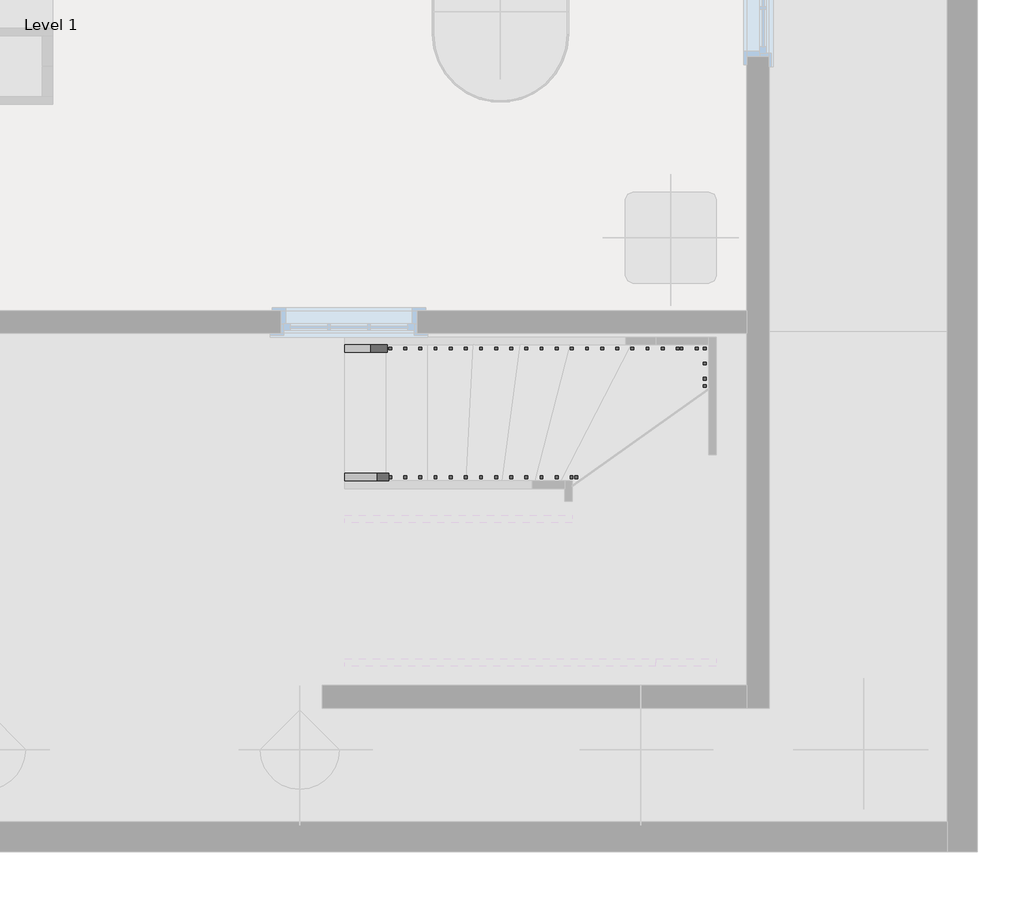
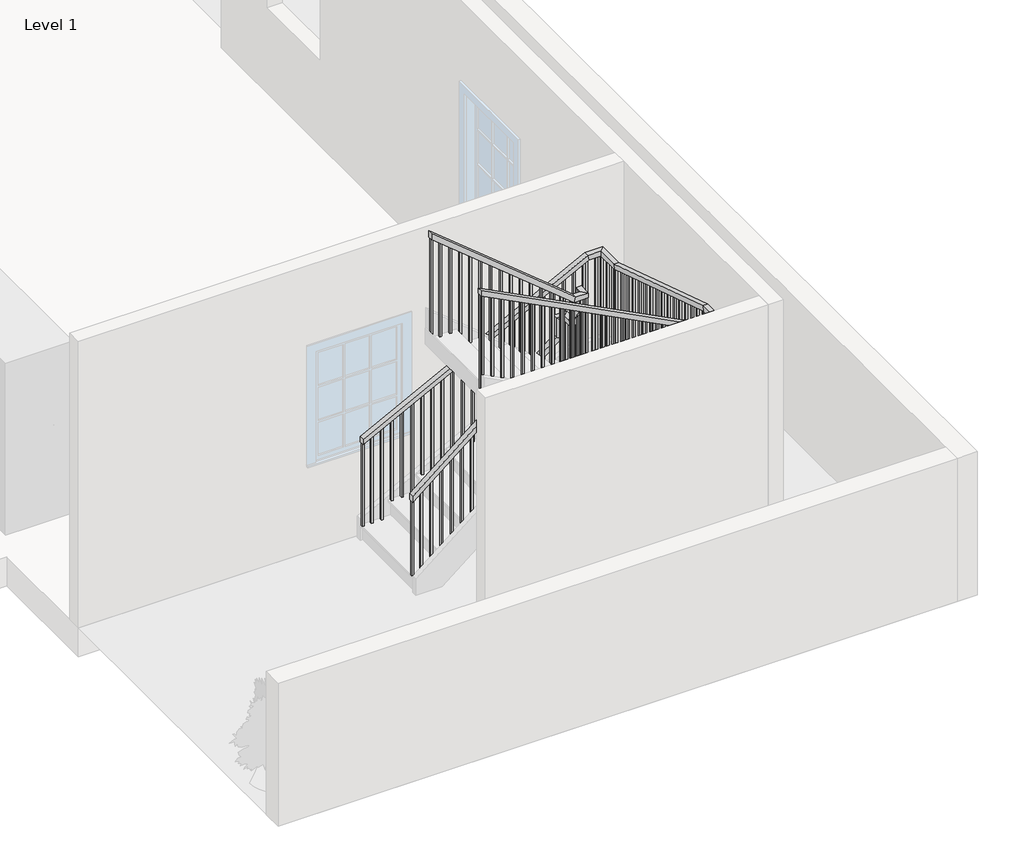
# One storey, part 2 of 3: 2 railings.
"""IFC4 building model written with IfcOpenShell, lengths in millimetres."""

from ifc_helpers import new_model, si_unit, frame, origin, place, context, project, spatial, polyline, outline, extrude, faceted_brep, element, save

model = new_model("IFC4")

# Units and contexts
model_context = context("Model", 3, world=origin())
ifc_project = project(units=[si_unit("LENGTHUNIT", "METRE", prefix="MILLI")], contexts=[model_context])

# Site, building, storey
site = spatial("IfcSite", under=ifc_project)
building = spatial("IfcBuilding", under=site)
storey = spatial("IfcBuildingStorey", under=building, Name="Level 1", Elevation=0.0)

# Railings
placement = place(None, origin())
element("IfcRailing", 1, ObjectType="Handrail - Rectangular", at=placement, inside=storey, context=model_context, shape_type="SolidModel", body=[
    faceted_brep([(-3966.7570938, 433.3007235, 1025.2529681), (-3966.7570938, 433.3007235, 959.7067088), (-3966.7570938, 382.5007235, 959.7067088), (-3966.7570938, 382.5007235, 1025.2529681), (-2515.2254019, 433.3007235, 2208.7848338), (-2464.4254019, 433.3007235, 2184.659247), (-2464.4254019, 382.5007235, 2184.659247), (-2515.2254019, 382.5007235, 2208.7848338), (-2515.2254019, 433.3007235, 2414.6281882), (-2464.4254019, 433.3007235, 2363.8281882), (-2464.4254019, 382.5007235, 2363.8281882), (-2515.2254019, 382.5007235, 2414.6281882), (-2388.2254019, 433.3007235, 2414.6281882), (-2388.2254019, 433.3007235, 2363.8281882), (-2439.0254019, 382.5007235, 2363.8281882), (-2439.0254019, 382.5007235, 2414.6281882), (-2388.2254019, 306.3007235, 2414.6281882), (-2388.2254019, 277.1793897, 2363.8281882), (-2439.0254019, 277.1793897, 2363.8281882), (-2439.0254019, 306.3007235, 2414.6281882), (-2388.2254019, 179.3007235, 2631.5051451), (-2388.2254019, 128.5007235, 2617.7256424), (-2439.0254019, 128.5007235, 2617.7256424), (-2439.0254019, 179.3007235, 2631.5051451), (-2388.2254019, 179.3007235, 2837.3484995), (-2388.2254019, 128.5007235, 2786.5484995), (-2439.0254019, 128.5007235, 2786.5484995), (-2439.0254019, 179.3007235, 2837.3484995), (-2388.2254019, 52.3007235, 2837.3484995), (-2388.2254019, 52.3007235, 2786.5484995), (-2439.0254019, 103.1007235, 2786.5484995), (-2439.0254019, 103.1007235, 2837.3484995), (-2515.2254019, 52.3007235, 2837.3484995), (-2533.310815, 52.3007235, 2786.5484995), (-2533.310815, 103.1007235, 2786.5484995), (-2515.2254019, 103.1007235, 2837.3484995), (-3966.7570938, 52.3007235, 4020.8803652), (-3966.7570938, 103.1007235, 4020.8803652), (-3966.7570938, 103.1007235, 3955.3341059), (-3966.7570938, 52.3007235, 3955.3341059)], [[[0, 1, 2, 3]], [[1, 0, 4, 5]], [[2, 1, 5, 6]], [[3, 2, 6, 7]], [[0, 3, 7, 4]], [[5, 4, 8, 9]], [[6, 5, 9, 10]], [[7, 6, 10, 11]], [[4, 7, 11, 8]], [[9, 8, 12, 13]], [[10, 9, 13, 14]], [[11, 10, 14, 15]], [[8, 11, 15, 12]], [[13, 12, 16, 17]], [[14, 13, 17, 18]], [[15, 14, 18, 19]], [[12, 15, 19, 16]], [[17, 16, 20, 21]], [[18, 17, 21, 22]], [[19, 18, 22, 23]], [[16, 19, 23, 20]], [[21, 20, 24, 25]], [[22, 21, 25, 26]], [[23, 22, 26, 27]], [[20, 23, 27, 24]], [[25, 24, 28, 29]], [[26, 25, 29, 30]], [[27, 26, 30, 31]], [[24, 27, 31, 28]], [[29, 28, 32, 33]], [[30, 29, 33, 34]], [[31, 30, 34, 35]], [[28, 31, 35, 32]], [[36, 37, 38, 39]], [[33, 32, 36, 39]], [[34, 33, 39, 38]], [[35, 34, 38, 37]], [[32, 35, 37, 36]]]),
    extrude(outline(polyline([(3866.2231262, -3857.4677583), (3881.7558784, -3876.5177583), (2878.6666667, -3876.5177583), (2878.6666667, -3857.4677583), (3866.2231262, -3857.4677583)])), frame((0.0, 68.1757235, 0.0), z_axis=(0.0, 1.0, 0.0), x_axis=(0.0, 0.0, 1.0)), (0.0, 0.0, 1.0), 19.05),
    extrude(outline(polyline([(3783.3817813, -3755.8677583), (3798.9145334, -3774.9177583), (2878.6666667, -3774.9177583), (2878.6666667, -3755.8677583), (3783.3817813, -3755.8677583)])), frame((0.0, 68.1757235, 0.0), z_axis=(0.0, 1.0, 0.0), x_axis=(0.0, 0.0, 1.0)), (0.0, 0.0, 1.0), 19.05),
    extrude(outline(polyline([(3700.5404364, -3654.2677583), (3716.0731885, -3673.3177583), (2709.3333333, -3673.3177583), (2709.3333333, -3654.2677583), (3700.5404364, -3654.2677583)])), frame((0.0, 68.1757235, 0.0), z_axis=(0.0, 1.0, 0.0), x_axis=(0.0, 0.0, 1.0)), (0.0, 0.0, 1.0), 19.05),
    extrude(outline(polyline([(3617.6990914, -3552.6677583), (3633.2318436, -3571.7177583), (2709.3333333, -3571.7177583), (2709.3333333, -3552.6677583), (3617.6990914, -3552.6677583)])), frame((0.0, 68.1757235, 0.0), z_axis=(0.0, 1.0, 0.0), x_axis=(0.0, 0.0, 1.0)), (0.0, 0.0, 1.0), 19.05),
    extrude(outline(polyline([(3534.8577465, -3451.0677583), (3550.3904987, -3470.1177583), (2709.3333333, -3470.1177583), (2709.3333333, -3451.0677583), (3534.8577465, -3451.0677583)])), frame((0.0, 68.1757235, 0.0), z_axis=(0.0, 1.0, 0.0), x_axis=(0.0, 0.0, 1.0)), (0.0, 0.0, 1.0), 19.05),
    extrude(outline(polyline([(3452.0164016, -3349.4677583), (3467.5491538, -3368.5177583), (2540.0, -3368.5177583), (2540.0, -3349.4677583), (3452.0164016, -3349.4677583)])), frame((0.0, 68.1757235, 0.0), z_axis=(0.0, 1.0, 0.0), x_axis=(0.0, 0.0, 1.0)), (0.0, 0.0, 1.0), 19.05),
    extrude(outline(polyline([(3369.1750567, -3247.8677583), (3384.7078088, -3266.9177583), (2540.0, -3266.9177583), (2540.0, -3247.8677583), (3369.1750567, -3247.8677583)])), frame((0.0, 68.1757235, 0.0), z_axis=(0.0, 1.0, 0.0), x_axis=(0.0, 0.0, 1.0)), (0.0, 0.0, 1.0), 19.05),
    extrude(outline(polyline([(3286.3337117, -3146.2677583), (3301.8664639, -3165.3177583), (2540.0, -3165.3177583), (2540.0, -3146.2677583), (3286.3337117, -3146.2677583)])), frame((0.0, 68.1757235, 0.0), z_axis=(0.0, 1.0, 0.0), x_axis=(0.0, 0.0, 1.0)), (0.0, 0.0, 1.0), 19.05),
    extrude(outline(polyline([(3203.4923668, -3044.6677583), (3219.025119, -3063.7177583), (2370.6666667, -3063.7177583), (2370.6666667, -3044.6677583), (3203.4923668, -3044.6677583)])), frame((0.0, 68.1757235, 0.0), z_axis=(0.0, 1.0, 0.0), x_axis=(0.0, 0.0, 1.0)), (0.0, 0.0, 1.0), 19.05),
    extrude(outline(polyline([(3120.6510219, -2943.0677583), (3136.1837741, -2962.1177583), (2370.6666667, -2962.1177583), (2370.6666667, -2943.0677583), (3120.6510219, -2943.0677583)])), frame((0.0, 68.1757235, 0.0), z_axis=(0.0, 1.0, 0.0), x_axis=(0.0, 0.0, 1.0)), (0.0, 0.0, 1.0), 19.05),
    extrude(outline(polyline([(3037.809677, -2841.4677583), (3053.3424291, -2860.5177583), (2201.3333333, -2860.5177583), (2201.3333333, -2841.4677583), (3037.809677, -2841.4677583)])), frame((0.0, 68.1757235, 0.0), z_axis=(0.0, 1.0, 0.0), x_axis=(0.0, 0.0, 1.0)), (0.0, 0.0, 1.0), 19.05),
    extrude(outline(polyline([(2954.9683321, -2739.8677583), (2970.5010842, -2758.9177583), (2201.3333333, -2758.9177583), (2201.3333333, -2739.8677583), (2954.9683321, -2739.8677583)])), frame((0.0, 68.1757235, 0.0), z_axis=(0.0, 1.0, 0.0), x_axis=(0.0, 0.0, 1.0)), (0.0, 0.0, 1.0), 19.05),
    extrude(outline(polyline([(2872.1269871, -2638.2677583), (2887.6597393, -2657.3177583), (2032.0, -2657.3177583), (2032.0, -2638.2677583), (2872.1269871, -2638.2677583)])), frame((0.0, 68.1757235, 0.0), z_axis=(0.0, 1.0, 0.0), x_axis=(0.0, 0.0, 1.0)), (0.0, 0.0, 1.0), 19.05),
    extrude(outline(polyline([(2789.2856422, -2536.6677583), (2804.8183944, -2555.7177583), (2032.0, -2555.7177583), (2032.0, -2536.6677583), (2789.2856422, -2536.6677583)])), frame((0.0, 68.1757235, 0.0), z_axis=(0.0, 1.0, 0.0), x_axis=(0.0, 0.0, 1.0)), (0.0, 0.0, 1.0), 19.05),
    extrude(outline(polyline([(180.3898197, 2529.115018), (199.4398197, 2496.5834745), (199.4398197, 1524.0), (180.3898197, 1524.0), (180.3898197, 2529.115018)])), frame((-2423.1504019, 0.0, 0.0), z_axis=(1.0, 0.0, 0.0), x_axis=(0.0, 1.0, 0.0)), (0.0, 0.0, 1.0), 19.05),
    extrude(outline(polyline([(281.9898197, 2355.6134525), (301.0398197, 2323.0819089), (301.0398197, 1524.0), (281.9898197, 1524.0), (281.9898197, 2355.6134525)])), frame((-2423.1504019, 0.0, 0.0), z_axis=(1.0, 0.0, 0.0), x_axis=(0.0, 1.0, 0.0)), (0.0, 0.0, 1.0), 19.05),
    extrude(outline(polyline([(2127.2519138, -2534.8320938), (2111.7191617, -2553.8820938), (1016.0, -2553.8820938), (1016.0, -2534.8320938), (2127.2519138, -2534.8320938)])), frame((0.0, 398.3757235, 0.0), z_axis=(0.0, 1.0, 0.0), x_axis=(0.0, 0.0, 1.0)), (0.0, 0.0, 1.0), 19.05),
    extrude(outline(polyline([(2044.4105689, -2636.4320938), (2028.8778167, -2655.4820938), (1016.0, -2655.4820938), (1016.0, -2636.4320938), (2044.4105689, -2636.4320938)])), frame((0.0, 398.3757235, 0.0), z_axis=(0.0, 1.0, 0.0), x_axis=(0.0, 0.0, 1.0)), (0.0, 0.0, 1.0), 19.05),
    extrude(outline(polyline([(1961.569224, -2738.0320938), (1946.0364718, -2757.0820938), (846.6666667, -2757.0820938), (846.6666667, -2738.0320938), (1961.569224, -2738.0320938)])), frame((0.0, 398.3757235, 0.0), z_axis=(0.0, 1.0, 0.0), x_axis=(0.0, 0.0, 1.0)), (0.0, 0.0, 1.0), 19.05),
    extrude(outline(polyline([(1878.7278791, -2839.6320938), (1863.1951269, -2858.6820938), (846.6666667, -2858.6820938), (846.6666667, -2839.6320938), (1878.7278791, -2839.6320938)])), frame((0.0, 398.3757235, 0.0), z_axis=(0.0, 1.0, 0.0), x_axis=(0.0, 0.0, 1.0)), (0.0, 0.0, 1.0), 19.05),
    extrude(outline(polyline([(1795.8865341, -2941.2320938), (1780.353782, -2960.2820938), (677.3333333, -2960.2820938), (677.3333333, -2941.2320938), (1795.8865341, -2941.2320938)])), frame((0.0, 398.3757235, 0.0), z_axis=(0.0, 1.0, 0.0), x_axis=(0.0, 0.0, 1.0)), (0.0, 0.0, 1.0), 19.05),
    extrude(outline(polyline([(1713.0451892, -3042.8320938), (1697.5124371, -3061.8820938), (677.3333333, -3061.8820938), (677.3333333, -3042.8320938), (1713.0451892, -3042.8320938)])), frame((0.0, 398.3757235, 0.0), z_axis=(0.0, 1.0, 0.0), x_axis=(0.0, 0.0, 1.0)), (0.0, 0.0, 1.0), 19.05),
    extrude(outline(polyline([(1630.2038443, -3144.4320938), (1614.6710921, -3163.4820938), (508.0, -3163.4820938), (508.0, -3144.4320938), (1630.2038443, -3144.4320938)])), frame((0.0, 398.3757235, 0.0), z_axis=(0.0, 1.0, 0.0), x_axis=(0.0, 0.0, 1.0)), (0.0, 0.0, 1.0), 19.05),
    extrude(outline(polyline([(1547.3624994, -3246.0320938), (1531.8297472, -3265.0820938), (508.0, -3265.0820938), (508.0, -3246.0320938), (1547.3624994, -3246.0320938)])), frame((0.0, 398.3757235, 0.0), z_axis=(0.0, 1.0, 0.0), x_axis=(0.0, 0.0, 1.0)), (0.0, 0.0, 1.0), 19.05),
    extrude(outline(polyline([(1464.5211545, -3347.6320938), (1448.9884023, -3366.6820938), (508.0, -3366.6820938), (508.0, -3347.6320938), (1464.5211545, -3347.6320938)])), frame((0.0, 398.3757235, 0.0), z_axis=(0.0, 1.0, 0.0), x_axis=(0.0, 0.0, 1.0)), (0.0, 0.0, 1.0), 19.05),
    extrude(outline(polyline([(1381.6798095, -3449.2320938), (1366.1470574, -3468.2820938), (338.6666667, -3468.2820938), (338.6666667, -3449.2320938), (1381.6798095, -3449.2320938)])), frame((0.0, 398.3757235, 0.0), z_axis=(0.0, 1.0, 0.0), x_axis=(0.0, 0.0, 1.0)), (0.0, 0.0, 1.0), 19.05),
    extrude(outline(polyline([(1298.8384646, -3550.8320938), (1283.3057124, -3569.8820938), (338.6666667, -3569.8820938), (338.6666667, -3550.8320938), (1298.8384646, -3550.8320938)])), frame((0.0, 398.3757235, 0.0), z_axis=(0.0, 1.0, 0.0), x_axis=(0.0, 0.0, 1.0)), (0.0, 0.0, 1.0), 19.05),
    extrude(outline(polyline([(1215.9971197, -3652.4320938), (1200.4643675, -3671.4820938), (338.6666667, -3671.4820938), (338.6666667, -3652.4320938), (1215.9971197, -3652.4320938)])), frame((0.0, 398.3757235, 0.0), z_axis=(0.0, 1.0, 0.0), x_axis=(0.0, 0.0, 1.0)), (0.0, 0.0, 1.0), 19.05),
    extrude(outline(polyline([(1133.1557748, -3754.0320938), (1117.6230226, -3773.0820938), (169.3333333, -3773.0820938), (169.3333333, -3754.0320938), (1133.1557748, -3754.0320938)])), frame((0.0, 398.3757235, 0.0), z_axis=(0.0, 1.0, 0.0), x_axis=(0.0, 0.0, 1.0)), (0.0, 0.0, 1.0), 19.05),
    extrude(outline(polyline([(1050.3144298, -3855.6320938), (1034.7816777, -3874.6820938), (169.3333333, -3874.6820938), (169.3333333, -3855.6320938), (1050.3144298, -3855.6320938)])), frame((0.0, 398.3757235, 0.0), z_axis=(0.0, 1.0, 0.0), x_axis=(0.0, 0.0, 1.0)), (0.0, 0.0, 1.0), 19.05),
    extrude(outline(polyline([(-2435.0677583, 87.2257235), (-2435.0677583, 68.1757235), (-2454.1177583, 68.1757235), (-2454.1177583, 87.2257235), (-2435.0677583, 87.2257235)])), frame((0.0, 0.0, 1862.6666667), z_axis=(0.0, 0.0, 1.0), x_axis=(1.0, 0.0, 0.0)), (0.0, 0.0, 1.0), 923.8818329),
    extrude(outline(polyline([(-2423.1504019, 87.2257235), (-2404.1004019, 87.2257235), (-2404.1004019, 68.1757235), (-2423.1504019, 68.1757235), (-2423.1504019, 87.2257235)])), frame((0.0, 0.0, 1862.6666667), z_axis=(0.0, 0.0, 1.0), x_axis=(1.0, 0.0, 0.0)), (0.0, 0.0, 1.0), 923.8818329),
    extrude(outline(polyline([(-2423.1504019, 102.0116273), (-2404.1004019, 102.0116273), (-2404.1004019, 82.9616273), (-2423.1504019, 82.9616273), (-2423.1504019, 102.0116273)])), frame((0.0, 0.0, 1693.3333333), z_axis=(0.0, 0.0, 1.0), x_axis=(1.0, 0.0, 0.0)), (0.0, 0.0, 1.0), 1093.2151662),
    extrude(outline(polyline([(-2423.1504019, 402.6398197), (-2404.1004019, 402.6398197), (-2404.1004019, 383.5898197), (-2423.1504019, 383.5898197), (-2423.1504019, 402.6398197)])), frame((0.0, 0.0, 1354.6666667), z_axis=(0.0, 0.0, 1.0), x_axis=(1.0, 0.0, 0.0)), (0.0, 0.0, 1.0), 1009.1615215),
    extrude(outline(polyline([(-2423.1504019, 398.3757235), (-2423.1504019, 417.4257235), (-2404.1004019, 417.4257235), (-2404.1004019, 398.3757235), (-2423.1504019, 398.3757235)])), frame((0.0, 0.0, 1185.3333333), z_axis=(0.0, 0.0, 1.0), x_axis=(1.0, 0.0, 0.0)), (0.0, 0.0, 1.0), 1178.4948549),
    extrude(outline(polyline([(-2454.1177583, 398.3757235), (-2454.1177583, 417.4257235), (-2435.0677583, 417.4257235), (-2435.0677583, 398.3757235), (-2454.1177583, 398.3757235)])), frame((0.0, 0.0, 1185.3333333), z_axis=(0.0, 0.0, 1.0), x_axis=(1.0, 0.0, 0.0)), (0.0, 0.0, 1.0), 1178.4948549),
    extrude(outline(polyline([(3939.8013537, -3947.7070938), (3955.3341059, -3966.7570938), (2878.6666667, -3966.7570938), (2878.6666667, -3947.7070938), (3939.8013537, -3947.7070938)])), frame((0.0, 68.1757235, 0.0), z_axis=(0.0, 1.0, 0.0), x_axis=(0.0, 0.0, 1.0)), (0.0, 0.0, 1.0), 19.05),
    extrude(outline(polyline([(975.239461, -3947.7070938), (959.7067088, -3966.7570938), (169.3333333, -3966.7570938), (169.3333333, -3947.7070938), (975.239461, -3947.7070938)])), frame((0.0, 398.3757235, 0.0), z_axis=(0.0, 1.0, 0.0), x_axis=(0.0, 0.0, 1.0)), (0.0, 0.0, 1.0), 19.05),
])
element("IfcRailing", 2, ObjectType="Handrail - Rectangular", at=placement, inside=storey, context=model_context, shape_type="SolidModel", body=[
    faceted_brep([(-3966.7570938, 1296.9007235, 1109.0771751), (-3966.7570938, 1296.9007235, 1051.9280057), (-3966.7570938, 1246.1007235, 1051.9280057), (-3966.7570938, 1246.1007235, 1109.0771751), (-1706.7752373, 1296.9007235, 2273.7644996), (-1694.455186, 1296.9007235, 2222.9644996), (-1694.455186, 1246.1007235, 2222.9644996), (-1706.7752373, 1246.1007235, 2273.7644996), (-1524.6254019, 1296.9007235, 2273.7644996), (-1524.6254019, 1296.9007235, 2222.9644996), (-1575.4254019, 1246.1007235, 2222.9644996), (-1575.4254019, 1246.1007235, 2273.7644996), (-1524.6254019, 1019.7467709, 2273.7644996), (-1524.6254019, 1011.7961947, 2222.9644996), (-1575.4254019, 1011.7961947, 2222.9644996), (-1575.4254019, 1019.7467709, 2273.7644996), (-1524.6254019, -534.1453239, 2772.3688337), (-1524.6254019, -542.0959, 2721.5688337), (-1575.4254019, -542.0959, 2721.5688337), (-1575.4254019, -534.1453239, 2772.3688337), (-1524.6254019, -811.2992765, 2772.3688337), (-1524.6254019, -811.2992765, 2721.5688337), (-1575.4254019, -760.4992765, 2721.5688337), (-1575.4254019, -760.4992765, 2772.3688337), (-1706.7752373, -811.2992765, 2772.3688337), (-1719.0952886, -811.2992765, 2721.5688337), (-1719.0952886, -760.4992765, 2721.5688337), (-1706.7752373, -760.4992765, 2772.3688337), (-3966.7570938, -811.2992765, 3937.0561582), (-3966.7570938, -760.4992765, 3937.0561582), (-3966.7570938, -760.4992765, 3879.9069889), (-3966.7570938, -811.2992765, 3879.9069889)], [[[0, 1, 2, 3]], [[1, 0, 4, 5]], [[2, 1, 5, 6]], [[3, 2, 6, 7]], [[0, 3, 7, 4]], [[5, 4, 8, 9]], [[6, 5, 9, 10]], [[7, 6, 10, 11]], [[4, 7, 11, 8]], [[9, 8, 12, 13]], [[10, 9, 13, 14]], [[11, 10, 14, 15]], [[8, 11, 15, 12]], [[13, 12, 16, 17]], [[14, 13, 17, 18]], [[15, 14, 18, 19]], [[12, 15, 19, 16]], [[17, 16, 20, 21]], [[18, 17, 21, 22]], [[19, 18, 22, 23]], [[16, 19, 23, 20]], [[21, 20, 24, 25]], [[22, 21, 25, 26]], [[23, 22, 26, 27]], [[20, 23, 27, 24]], [[28, 29, 30, 31]], [[25, 24, 28, 31]], [[26, 25, 31, 30]], [[27, 26, 30, 29]], [[24, 27, 29, 28]]]),
    extrude(outline(polyline([(3872.0443296, -3951.5002373), (2878.6666667, -3951.5002373), (2878.6666667, -3932.4502373), (3862.2268642, -3932.4502373), (3872.0443296, -3951.5002373)])), frame((0.0, -795.4242765, 0.0), z_axis=(0.0, 1.0, 0.0), x_axis=(0.0, 0.0, 1.0)), (0.0, 0.0, 1.0), 19.05),
    extrude(outline(polyline([(3819.6845145, -3849.9002373), (2878.6666667, -3849.9002373), (2878.6666667, -3830.8502373), (3809.8670491, -3830.8502373), (3819.6845145, -3849.9002373)])), frame((0.0, -795.4242765, 0.0), z_axis=(0.0, 1.0, 0.0), x_axis=(0.0, 0.0, 1.0)), (0.0, 0.0, 1.0), 19.05),
    extrude(outline(polyline([(3767.3246993, -3748.3002373), (2878.6666667, -3748.3002373), (2878.6666667, -3729.2502373), (3757.507234, -3729.2502373), (3767.3246993, -3748.3002373)])), frame((0.0, -795.4242765, 0.0), z_axis=(0.0, 1.0, 0.0), x_axis=(0.0, 0.0, 1.0)), (0.0, 0.0, 1.0), 19.05),
    extrude(outline(polyline([(3714.9648842, -3646.7002373), (2709.3333333, -3646.7002373), (2709.3333333, -3627.6502373), (3705.1474189, -3627.6502373), (3714.9648842, -3646.7002373)])), frame((0.0, -795.4242765, 0.0), z_axis=(0.0, 1.0, 0.0), x_axis=(0.0, 0.0, 1.0)), (0.0, 0.0, 1.0), 19.05),
    extrude(outline(polyline([(3662.6050691, -3545.1002373), (2709.3333333, -3545.1002373), (2709.3333333, -3526.0502373), (3652.7876038, -3526.0502373), (3662.6050691, -3545.1002373)])), frame((0.0, -795.4242765, 0.0), z_axis=(0.0, 1.0, 0.0), x_axis=(0.0, 0.0, 1.0)), (0.0, 0.0, 1.0), 19.05),
    extrude(outline(polyline([(3610.245254, -3443.5002373), (2709.3333333, -3443.5002373), (2709.3333333, -3424.4502373), (3600.4277887, -3424.4502373), (3610.245254, -3443.5002373)])), frame((0.0, -795.4242765, 0.0), z_axis=(0.0, 1.0, 0.0), x_axis=(0.0, 0.0, 1.0)), (0.0, 0.0, 1.0), 19.05),
    extrude(outline(polyline([(3557.8854389, -3341.9002373), (2540.0, -3341.9002373), (2540.0, -3322.8502373), (3548.0679735, -3322.8502373), (3557.8854389, -3341.9002373)])), frame((0.0, -795.4242765, 0.0), z_axis=(0.0, 1.0, 0.0), x_axis=(0.0, 0.0, 1.0)), (0.0, 0.0, 1.0), 19.05),
    extrude(outline(polyline([(3505.5256238, -3240.3002373), (2540.0, -3240.3002373), (2540.0, -3221.2502373), (3495.7081584, -3221.2502373), (3505.5256238, -3240.3002373)])), frame((0.0, -795.4242765, 0.0), z_axis=(0.0, 1.0, 0.0), x_axis=(0.0, 0.0, 1.0)), (0.0, 0.0, 1.0), 19.05),
    extrude(outline(polyline([(3453.1658086, -3138.7002373), (2540.0, -3138.7002373), (2540.0, -3119.6502373), (3443.3483433, -3119.6502373), (3453.1658086, -3138.7002373)])), frame((0.0, -795.4242765, 0.0), z_axis=(0.0, 1.0, 0.0), x_axis=(0.0, 0.0, 1.0)), (0.0, 0.0, 1.0), 19.05),
    extrude(outline(polyline([(3400.8059935, -3037.1002373), (2370.6666667, -3037.1002373), (2370.6666667, -3018.0502373), (3390.9885282, -3018.0502373), (3400.8059935, -3037.1002373)])), frame((0.0, -795.4242765, 0.0), z_axis=(0.0, 1.0, 0.0), x_axis=(0.0, 0.0, 1.0)), (0.0, 0.0, 1.0), 19.05),
    extrude(outline(polyline([(3348.4461784, -2935.5002373), (2370.6666667, -2935.5002373), (2370.6666667, -2916.4502373), (3338.6287131, -2916.4502373), (3348.4461784, -2935.5002373)])), frame((0.0, -795.4242765, 0.0), z_axis=(0.0, 1.0, 0.0), x_axis=(0.0, 0.0, 1.0)), (0.0, 0.0, 1.0), 19.05),
    extrude(outline(polyline([(3296.0863633, -2833.9002373), (2370.6666667, -2833.9002373), (2370.6666667, -2814.8502373), (3286.268898, -2814.8502373), (3296.0863633, -2833.9002373)])), frame((0.0, -795.4242765, 0.0), z_axis=(0.0, 1.0, 0.0), x_axis=(0.0, 0.0, 1.0)), (0.0, 0.0, 1.0), 19.05),
    extrude(outline(polyline([(3243.7265482, -2732.3002373), (2201.3333333, -2732.3002373), (2201.3333333, -2713.2502373), (3233.9090828, -2713.2502373), (3243.7265482, -2732.3002373)])), frame((0.0, -795.4242765, 0.0), z_axis=(0.0, 1.0, 0.0), x_axis=(0.0, 0.0, 1.0)), (0.0, 0.0, 1.0), 19.05),
    extrude(outline(polyline([(3191.3667331, -2630.7002373), (2201.3333333, -2630.7002373), (2201.3333333, -2611.6502373), (3181.5492677, -2611.6502373), (3191.3667331, -2630.7002373)])), frame((0.0, -795.4242765, 0.0), z_axis=(0.0, 1.0, 0.0), x_axis=(0.0, 0.0, 1.0)), (0.0, 0.0, 1.0), 19.05),
    extrude(outline(polyline([(3139.0069179, -2529.1002373), (2201.3333333, -2529.1002373), (2201.3333333, -2510.0502373), (3129.1894526, -2510.0502373), (3139.0069179, -2529.1002373)])), frame((0.0, -795.4242765, 0.0), z_axis=(0.0, 1.0, 0.0), x_axis=(0.0, 0.0, 1.0)), (0.0, 0.0, 1.0), 19.05),
    extrude(outline(polyline([(3086.6471028, -2427.5002373), (2032.0, -2427.5002373), (2032.0, -2408.4502373), (3076.8296375, -2408.4502373), (3086.6471028, -2427.5002373)])), frame((0.0, -795.4242765, 0.0), z_axis=(0.0, 1.0, 0.0), x_axis=(0.0, 0.0, 1.0)), (0.0, 0.0, 1.0), 19.05),
    extrude(outline(polyline([(3034.2872877, -2325.9002373), (2032.0, -2325.9002373), (2032.0, -2306.8502373), (3024.4698224, -2306.8502373), (3034.2872877, -2325.9002373)])), frame((0.0, -795.4242765, 0.0), z_axis=(0.0, 1.0, 0.0), x_axis=(0.0, 0.0, 1.0)), (0.0, 0.0, 1.0), 19.05),
    extrude(outline(polyline([(2981.9274726, -2224.3002373), (2032.0, -2224.3002373), (2032.0, -2205.2502373), (2972.1100073, -2205.2502373), (2981.9274726, -2224.3002373)])), frame((0.0, -795.4242765, 0.0), z_axis=(0.0, 1.0, 0.0), x_axis=(0.0, 0.0, 1.0)), (0.0, 0.0, 1.0), 19.05),
    extrude(outline(polyline([(2929.5676575, -2122.7002373), (2032.0, -2122.7002373), (2032.0, -2103.6502373), (2919.7501921, -2103.6502373), (2929.5676575, -2122.7002373)])), frame((0.0, -795.4242765, 0.0), z_axis=(0.0, 1.0, 0.0), x_axis=(0.0, 0.0, 1.0)), (0.0, 0.0, 1.0), 19.05),
    extrude(outline(polyline([(2877.2078424, -2021.1002373), (1862.6666667, -2021.1002373), (1862.6666667, -2002.0502373), (2867.390377, -2002.0502373), (2877.2078424, -2021.1002373)])), frame((0.0, -795.4242765, 0.0), z_axis=(0.0, 1.0, 0.0), x_axis=(0.0, 0.0, 1.0)), (0.0, 0.0, 1.0), 19.05),
    extrude(outline(polyline([(2824.8480272, -1919.5002373), (1862.6666667, -1919.5002373), (1862.6666667, -1900.4502373), (2815.0305619, -1900.4502373), (2824.8480272, -1919.5002373)])), frame((0.0, -795.4242765, 0.0), z_axis=(0.0, 1.0, 0.0), x_axis=(0.0, 0.0, 1.0)), (0.0, 0.0, 1.0), 19.05),
    extrude(outline(polyline([(2772.4882121, -1817.9002373), (1862.6666667, -1817.9002373), (1862.6666667, -1798.8502373), (2762.6707468, -1798.8502373), (2772.4882121, -1817.9002373)])), frame((0.0, -795.4242765, 0.0), z_axis=(0.0, 1.0, 0.0), x_axis=(0.0, 0.0, 1.0)), (0.0, 0.0, 1.0), 19.05),
    extrude(outline(polyline([(-1642.1004019, -795.4242765), (-1661.1504019, -795.4242765), (-1661.1504019, -776.3742765), (-1642.1004019, -776.3742765), (-1642.1004019, -795.4242765)])), frame((0.0, 0.0, 1862.6666667), z_axis=(0.0, 0.0, 1.0), x_axis=(1.0, 0.0, 0.0)), (0.0, 0.0, 1.0), 858.902167),
    extrude(outline(polyline([(-1540.5004019, -727.8203239), (-1540.5004019, -746.8703239), (-1559.5504019, -746.8703239), (-1559.5504019, -727.8203239), (-1540.5004019, -727.8203239)])), frame((0.0, 0.0, 1862.6666667), z_axis=(0.0, 0.0, 1.0), x_axis=(1.0, 0.0, 0.0)), (0.0, 0.0, 1.0), 858.902167),
    extrude(outline(polyline([(-1540.5004019, -626.2203239), (-1540.5004019, -645.2703239), (-1559.5504019, -645.2703239), (-1559.5504019, -626.2203239), (-1540.5004019, -626.2203239)])), frame((0.0, 0.0, 1862.6666667), z_axis=(0.0, 0.0, 1.0), x_axis=(1.0, 0.0, 0.0)), (0.0, 0.0, 1.0), 858.902167),
    extrude(outline(polyline([(-494.7282291, 2706.3697564), (-494.7282291, 1693.3333333), (-513.7782291, 1693.3333333), (-513.7782291, 2712.4824155), (-494.7282291, 2706.3697564)])), frame((-1559.5504019, 0.0, 0.0), z_axis=(1.0, 0.0, 0.0), x_axis=(0.0, 1.0, 0.0)), (0.0, 0.0, 1.0), 19.05),
    extrude(outline(polyline([(-393.1282291, 2673.7689082), (-393.1282291, 1693.3333333), (-412.1782291, 1693.3333333), (-412.1782291, 2679.8815673), (-393.1282291, 2673.7689082)])), frame((-1559.5504019, 0.0, 0.0), z_axis=(1.0, 0.0, 0.0), x_axis=(0.0, 1.0, 0.0)), (0.0, 0.0, 1.0), 19.05),
    extrude(outline(polyline([(-291.5282291, 2641.16806), (-291.5282291, 1693.3333333), (-310.5782291, 1693.3333333), (-310.5782291, 2647.280719), (-291.5282291, 2641.16806)])), frame((-1559.5504019, 0.0, 0.0), z_axis=(1.0, 0.0, 0.0), x_axis=(0.0, 1.0, 0.0)), (0.0, 0.0, 1.0), 19.05),
    extrude(outline(polyline([(-189.9282291, 2608.5672118), (-189.9282291, 1693.3333333), (-208.9782291, 1693.3333333), (-208.9782291, 2614.6798708), (-189.9282291, 2608.5672118)])), frame((-1559.5504019, 0.0, 0.0), z_axis=(1.0, 0.0, 0.0), x_axis=(0.0, 1.0, 0.0)), (0.0, 0.0, 1.0), 19.05),
    extrude(outline(polyline([(-88.3282291, 2575.9663635), (-88.3282291, 1693.3333333), (-107.3782291, 1693.3333333), (-107.3782291, 2582.0790226), (-88.3282291, 2575.9663635)])), frame((-1559.5504019, 0.0, 0.0), z_axis=(1.0, 0.0, 0.0), x_axis=(0.0, 1.0, 0.0)), (0.0, 0.0, 1.0), 19.05),
    extrude(outline(polyline([(13.2717709, 2543.3655153), (13.2717709, 1693.3333333), (-5.7782291, 1693.3333333), (-5.7782291, 2549.4781744), (13.2717709, 2543.3655153)])), frame((-1559.5504019, 0.0, 0.0), z_axis=(1.0, 0.0, 0.0), x_axis=(0.0, 1.0, 0.0)), (0.0, 0.0, 1.0), 19.05),
    extrude(outline(polyline([(114.8717709, 2510.7646671), (114.8717709, 1524.0), (95.8217709, 1524.0), (95.8217709, 2516.8773261), (114.8717709, 2510.7646671)])), frame((-1559.5504019, 0.0, 0.0), z_axis=(1.0, 0.0, 0.0), x_axis=(0.0, 1.0, 0.0)), (0.0, 0.0, 1.0), 19.05),
    extrude(outline(polyline([(216.4717709, 2478.1638189), (216.4717709, 1524.0), (197.4217709, 1524.0), (197.4217709, 2484.2764779), (216.4717709, 2478.1638189)])), frame((-1559.5504019, 0.0, 0.0), z_axis=(1.0, 0.0, 0.0), x_axis=(0.0, 1.0, 0.0)), (0.0, 0.0, 1.0), 19.05),
    extrude(outline(polyline([(318.0717709, 2445.5629706), (318.0717709, 1524.0), (299.0217709, 1524.0), (299.0217709, 2451.6756297), (318.0717709, 2445.5629706)])), frame((-1559.5504019, 0.0, 0.0), z_axis=(1.0, 0.0, 0.0), x_axis=(0.0, 1.0, 0.0)), (0.0, 0.0, 1.0), 19.05),
    extrude(outline(polyline([(419.6717709, 2412.9621224), (419.6717709, 1524.0), (400.6217709, 1524.0), (400.6217709, 2419.0747814), (419.6717709, 2412.9621224)])), frame((-1559.5504019, 0.0, 0.0), z_axis=(1.0, 0.0, 0.0), x_axis=(0.0, 1.0, 0.0)), (0.0, 0.0, 1.0), 19.05),
    extrude(outline(polyline([(521.2717709, 2380.3612742), (521.2717709, 1354.6666667), (502.2217709, 1354.6666667), (502.2217709, 2386.4739332), (521.2717709, 2380.3612742)])), frame((-1559.5504019, 0.0, 0.0), z_axis=(1.0, 0.0, 0.0), x_axis=(0.0, 1.0, 0.0)), (0.0, 0.0, 1.0), 19.05),
    extrude(outline(polyline([(622.8717709, 2347.7604259), (622.8717709, 1354.6666667), (603.8217709, 1354.6666667), (603.8217709, 2353.873085), (622.8717709, 2347.7604259)])), frame((-1559.5504019, 0.0, 0.0), z_axis=(1.0, 0.0, 0.0), x_axis=(0.0, 1.0, 0.0)), (0.0, 0.0, 1.0), 19.05),
    extrude(outline(polyline([(724.4717709, 2315.1595777), (724.4717709, 1354.6666667), (705.4217709, 1354.6666667), (705.4217709, 2321.2722368), (724.4717709, 2315.1595777)])), frame((-1559.5504019, 0.0, 0.0), z_axis=(1.0, 0.0, 0.0), x_axis=(0.0, 1.0, 0.0)), (0.0, 0.0, 1.0), 19.05),
    extrude(outline(polyline([(826.0717709, 2282.5587295), (826.0717709, 1354.6666667), (807.0217709, 1354.6666667), (807.0217709, 2288.6713885), (826.0717709, 2282.5587295)])), frame((-1559.5504019, 0.0, 0.0), z_axis=(1.0, 0.0, 0.0), x_axis=(0.0, 1.0, 0.0)), (0.0, 0.0, 1.0), 19.05),
    extrude(outline(polyline([(927.6717709, 2249.9578813), (927.6717709, 1354.6666667), (908.6217709, 1354.6666667), (908.6217709, 2256.0705403), (927.6717709, 2249.9578813)])), frame((-1559.5504019, 0.0, 0.0), z_axis=(1.0, 0.0, 0.0), x_axis=(0.0, 1.0, 0.0)), (0.0, 0.0, 1.0), 19.05),
    extrude(outline(polyline([(-1540.5004019, 1077.8257235), (-1540.5004019, 1058.7757235), (-1559.5504019, 1058.7757235), (-1559.5504019, 1077.8257235), (-1540.5004019, 1077.8257235)])), frame((0.0, 0.0, 1185.3333333), z_axis=(0.0, 0.0, 1.0), x_axis=(1.0, 0.0, 0.0)), (0.0, 0.0, 1.0), 1037.6311663),
    extrude(outline(polyline([(-1540.5004019, 1179.4257235), (-1540.5004019, 1160.3757235), (-1559.5504019, 1160.3757235), (-1559.5504019, 1179.4257235), (-1540.5004019, 1179.4257235)])), frame((0.0, 0.0, 1185.3333333), z_axis=(0.0, 0.0, 1.0), x_axis=(1.0, 0.0, 0.0)), (0.0, 0.0, 1.0), 1037.6311663),
    extrude(outline(polyline([(-1614.7002373, 1281.0257235), (-1595.6502373, 1281.0257235), (-1595.6502373, 1261.9757235), (-1614.7002373, 1261.9757235), (-1614.7002373, 1281.0257235)])), frame((0.0, 0.0, 1185.3333333), z_axis=(0.0, 0.0, 1.0), x_axis=(1.0, 0.0, 0.0)), (0.0, 0.0, 1.0), 1037.6311663),
    extrude(outline(polyline([(2198.9352056, -1741.0820938), (1185.3333333, -1741.0820938), (1185.3333333, -1722.0320938), (2208.752671, -1722.0320938), (2198.9352056, -1741.0820938)])), frame((0.0, 1261.9757235, 0.0), z_axis=(0.0, 1.0, 0.0), x_axis=(0.0, 0.0, 1.0)), (0.0, 0.0, 1.0), 19.05),
    extrude(outline(polyline([(2146.5753905, -1842.6820938), (1185.3333333, -1842.6820938), (1185.3333333, -1823.6320938), (2156.3928558, -1823.6320938), (2146.5753905, -1842.6820938)])), frame((0.0, 1261.9757235, 0.0), z_axis=(0.0, 1.0, 0.0), x_axis=(0.0, 0.0, 1.0)), (0.0, 0.0, 1.0), 19.05),
    extrude(outline(polyline([(2094.2155754, -1944.2820938), (1185.3333333, -1944.2820938), (1185.3333333, -1925.2320938), (2104.0330407, -1925.2320938), (2094.2155754, -1944.2820938)])), frame((0.0, 1261.9757235, 0.0), z_axis=(0.0, 1.0, 0.0), x_axis=(0.0, 0.0, 1.0)), (0.0, 0.0, 1.0), 19.05),
    extrude(outline(polyline([(2041.8557603, -2045.8820938), (1185.3333333, -2045.8820938), (1185.3333333, -2026.8320938), (2051.6732256, -2026.8320938), (2041.8557603, -2045.8820938)])), frame((0.0, 1261.9757235, 0.0), z_axis=(0.0, 1.0, 0.0), x_axis=(0.0, 0.0, 1.0)), (0.0, 0.0, 1.0), 19.05),
    extrude(outline(polyline([(1989.4959452, -2147.4820938), (1016.0, -2147.4820938), (1016.0, -2128.4320938), (1999.3134105, -2128.4320938), (1989.4959452, -2147.4820938)])), frame((0.0, 1261.9757235, 0.0), z_axis=(0.0, 1.0, 0.0), x_axis=(0.0, 0.0, 1.0)), (0.0, 0.0, 1.0), 19.05),
    extrude(outline(polyline([(1937.13613, -2249.0820938), (1016.0, -2249.0820938), (1016.0, -2230.0320938), (1946.9535954, -2230.0320938), (1937.13613, -2249.0820938)])), frame((0.0, 1261.9757235, 0.0), z_axis=(0.0, 1.0, 0.0), x_axis=(0.0, 0.0, 1.0)), (0.0, 0.0, 1.0), 19.05),
    extrude(outline(polyline([(1884.7763149, -2350.6820938), (1016.0, -2350.6820938), (1016.0, -2331.6320938), (1894.5937803, -2331.6320938), (1884.7763149, -2350.6820938)])), frame((0.0, 1261.9757235, 0.0), z_axis=(0.0, 1.0, 0.0), x_axis=(0.0, 0.0, 1.0)), (0.0, 0.0, 1.0), 19.05),
    extrude(outline(polyline([(1832.4164998, -2452.2820938), (1016.0, -2452.2820938), (1016.0, -2433.2320938), (1842.2339651, -2433.2320938), (1832.4164998, -2452.2820938)])), frame((0.0, 1261.9757235, 0.0), z_axis=(0.0, 1.0, 0.0), x_axis=(0.0, 0.0, 1.0)), (0.0, 0.0, 1.0), 19.05),
    extrude(outline(polyline([(1780.0566847, -2553.8820938), (846.6666667, -2553.8820938), (846.6666667, -2534.8320938), (1789.87415, -2534.8320938), (1780.0566847, -2553.8820938)])), frame((0.0, 1261.9757235, 0.0), z_axis=(0.0, 1.0, 0.0), x_axis=(0.0, 0.0, 1.0)), (0.0, 0.0, 1.0), 19.05),
    extrude(outline(polyline([(1727.6968696, -2655.4820938), (846.6666667, -2655.4820938), (846.6666667, -2636.4320938), (1737.5143349, -2636.4320938), (1727.6968696, -2655.4820938)])), frame((0.0, 1261.9757235, 0.0), z_axis=(0.0, 1.0, 0.0), x_axis=(0.0, 0.0, 1.0)), (0.0, 0.0, 1.0), 19.05),
    extrude(outline(polyline([(1675.3370545, -2757.0820938), (846.6666667, -2757.0820938), (846.6666667, -2738.0320938), (1685.1545198, -2738.0320938), (1675.3370545, -2757.0820938)])), frame((0.0, 1261.9757235, 0.0), z_axis=(0.0, 1.0, 0.0), x_axis=(0.0, 0.0, 1.0)), (0.0, 0.0, 1.0), 19.05),
    extrude(outline(polyline([(1622.9772393, -2858.6820938), (677.3333333, -2858.6820938), (677.3333333, -2839.6320938), (1632.7947047, -2839.6320938), (1622.9772393, -2858.6820938)])), frame((0.0, 1261.9757235, 0.0), z_axis=(0.0, 1.0, 0.0), x_axis=(0.0, 0.0, 1.0)), (0.0, 0.0, 1.0), 19.05),
    extrude(outline(polyline([(1570.6174242, -2960.2820938), (677.3333333, -2960.2820938), (677.3333333, -2941.2320938), (1580.4348896, -2941.2320938), (1570.6174242, -2960.2820938)])), frame((0.0, 1261.9757235, 0.0), z_axis=(0.0, 1.0, 0.0), x_axis=(0.0, 0.0, 1.0)), (0.0, 0.0, 1.0), 19.05),
    extrude(outline(polyline([(1518.2576091, -3061.8820938), (677.3333333, -3061.8820938), (677.3333333, -3042.8320938), (1528.0750744, -3042.8320938), (1518.2576091, -3061.8820938)])), frame((0.0, 1261.9757235, 0.0), z_axis=(0.0, 1.0, 0.0), x_axis=(0.0, 0.0, 1.0)), (0.0, 0.0, 1.0), 19.05),
    extrude(outline(polyline([(1465.897794, -3163.4820938), (508.0, -3163.4820938), (508.0, -3144.4320938), (1475.7152593, -3144.4320938), (1465.897794, -3163.4820938)])), frame((0.0, 1261.9757235, 0.0), z_axis=(0.0, 1.0, 0.0), x_axis=(0.0, 0.0, 1.0)), (0.0, 0.0, 1.0), 19.05),
    extrude(outline(polyline([(1413.5379789, -3265.0820938), (508.0, -3265.0820938), (508.0, -3246.0320938), (1423.3554442, -3246.0320938), (1413.5379789, -3265.0820938)])), frame((0.0, 1261.9757235, 0.0), z_axis=(0.0, 1.0, 0.0), x_axis=(0.0, 0.0, 1.0)), (0.0, 0.0, 1.0), 19.05),
    extrude(outline(polyline([(1361.1781638, -3366.6820938), (508.0, -3366.6820938), (508.0, -3347.6320938), (1370.9956291, -3347.6320938), (1361.1781638, -3366.6820938)])), frame((0.0, 1261.9757235, 0.0), z_axis=(0.0, 1.0, 0.0), x_axis=(0.0, 0.0, 1.0)), (0.0, 0.0, 1.0), 19.05),
    extrude(outline(polyline([(1308.8183486, -3468.2820938), (338.6666667, -3468.2820938), (338.6666667, -3449.2320938), (1318.635814, -3449.2320938), (1308.8183486, -3468.2820938)])), frame((0.0, 1261.9757235, 0.0), z_axis=(0.0, 1.0, 0.0), x_axis=(0.0, 0.0, 1.0)), (0.0, 0.0, 1.0), 19.05),
    extrude(outline(polyline([(1256.4585335, -3569.8820938), (338.6666667, -3569.8820938), (338.6666667, -3550.8320938), (1266.2759989, -3550.8320938), (1256.4585335, -3569.8820938)])), frame((0.0, 1261.9757235, 0.0), z_axis=(0.0, 1.0, 0.0), x_axis=(0.0, 0.0, 1.0)), (0.0, 0.0, 1.0), 19.05),
    extrude(outline(polyline([(1204.0987184, -3671.4820938), (338.6666667, -3671.4820938), (338.6666667, -3652.4320938), (1213.9161837, -3652.4320938), (1204.0987184, -3671.4820938)])), frame((0.0, 1261.9757235, 0.0), z_axis=(0.0, 1.0, 0.0), x_axis=(0.0, 0.0, 1.0)), (0.0, 0.0, 1.0), 19.05),
    extrude(outline(polyline([(1151.7389033, -3773.0820938), (169.3333333, -3773.0820938), (169.3333333, -3754.0320938), (1161.5563686, -3754.0320938), (1151.7389033, -3773.0820938)])), frame((0.0, 1261.9757235, 0.0), z_axis=(0.0, 1.0, 0.0), x_axis=(0.0, 0.0, 1.0)), (0.0, 0.0, 1.0), 19.05),
    extrude(outline(polyline([(1099.3790882, -3874.6820938), (169.3333333, -3874.6820938), (169.3333333, -3855.6320938), (1109.1965535, -3855.6320938), (1099.3790882, -3874.6820938)])), frame((0.0, 1261.9757235, 0.0), z_axis=(0.0, 1.0, 0.0), x_axis=(0.0, 0.0, 1.0)), (0.0, 0.0, 1.0), 19.05),
    extrude(outline(polyline([(-1697.2502373, -795.4242765), (-1716.3002373, -795.4242765), (-1716.3002373, -776.3742765), (-1697.2502373, -776.3742765), (-1697.2502373, -795.4242765)])), frame((0.0, 0.0, 1862.6666667), z_axis=(0.0, 0.0, 1.0), x_axis=(1.0, 0.0, 0.0)), (0.0, 0.0, 1.0), 858.902167),
    extrude(outline(polyline([(-1540.5004019, -776.3742765), (-1540.5004019, -795.4242765), (-1559.5504019, -795.4242765), (-1559.5504019, -776.3742765), (-1540.5004019, -776.3742765)])), frame((0.0, 0.0, 1862.6666667), z_axis=(0.0, 0.0, 1.0), x_axis=(1.0, 0.0, 0.0)), (0.0, 0.0, 1.0), 858.902167),
    extrude(outline(polyline([(-524.6203239, 2715.9613671), (-524.6203239, 1862.6666667), (-543.6703239, 1862.6666667), (-543.6703239, 2722.0740262), (-524.6203239, 2715.9613671)])), frame((-1559.5504019, 0.0, 0.0), z_axis=(1.0, 0.0, 0.0), x_axis=(0.0, 1.0, 0.0)), (0.0, 0.0, 1.0), 19.05),
    extrude(outline(polyline([(-1540.5004019, 1029.2717709), (-1540.5004019, 1010.2217709), (-1559.5504019, 1010.2217709), (-1559.5504019, 1029.2717709), (-1540.5004019, 1029.2717709)])), frame((0.0, 0.0, 1185.3333333), z_axis=(0.0, 0.0, 1.0), x_axis=(1.0, 0.0, 0.0)), (0.0, 0.0, 1.0), 1037.6311663),
    extrude(outline(polyline([(-1559.5504019, 1281.0257235), (-1540.5004019, 1281.0257235), (-1540.5004019, 1261.9757235), (-1559.5504019, 1261.9757235), (-1559.5504019, 1281.0257235)])), frame((0.0, 0.0, 1185.3333333), z_axis=(0.0, 0.0, 1.0), x_axis=(1.0, 0.0, 0.0)), (0.0, 0.0, 1.0), 1037.6311663),
    extrude(outline(polyline([(2211.7065976, -1716.3002373), (1185.3333333, -1716.3002373), (1185.3333333, -1697.2502373), (2221.5240629, -1697.2502373), (2211.7065976, -1716.3002373)])), frame((0.0, 1261.9757235, 0.0), z_axis=(0.0, 1.0, 0.0), x_axis=(0.0, 0.0, 1.0)), (0.0, 0.0, 1.0), 19.05),
    extrude(outline(polyline([(3879.9069889, -3966.7570938), (2878.6666667, -3966.7570938), (2878.6666667, -3947.7070938), (3870.0895235, -3947.7070938), (3879.9069889, -3966.7570938)])), frame((0.0, -795.4242765, 0.0), z_axis=(0.0, 1.0, 0.0), x_axis=(0.0, 0.0, 1.0)), (0.0, 0.0, 1.0), 19.05),
    extrude(outline(polyline([(1051.9280057, -3966.7570938), (169.3333333, -3966.7570938), (169.3333333, -3947.7070938), (1061.7454711, -3947.7070938), (1051.9280057, -3966.7570938)])), frame((0.0, 1261.9757235, 0.0), z_axis=(0.0, 1.0, 0.0), x_axis=(0.0, 0.0, 1.0)), (0.0, 0.0, 1.0), 19.05),
])

save(model, "model.ifc")

# Revit data of these elements
# Type "Handrail - Rectangular"
#   Assembly Code = "C2010400"
#   built-in parameter 1008612 = 0.0416667 (stored number, unit not read)
#   built-in parameter 1008611 = 0.0416667 (stored number, unit not read)
#   built-in parameter 1008609 = 0.333333 (stored number, unit not read)
#   built-in parameter 1008604 = 0.166667 (stored number, unit not read)
#   built-in parameter 1008603 = 0.166667 (stored number, unit not read)
#   Railing Height = 3' - 0"
#   built-in parameter 1008630 = 2
#   built-in parameter 1008610 = 2
#   built-in parameter 1008618 = Baluster - Square : 3/4"
# Elements 1, 2 (IfcRailing, "Handrail - Rectangular")
#   Phase Created = New Construction
